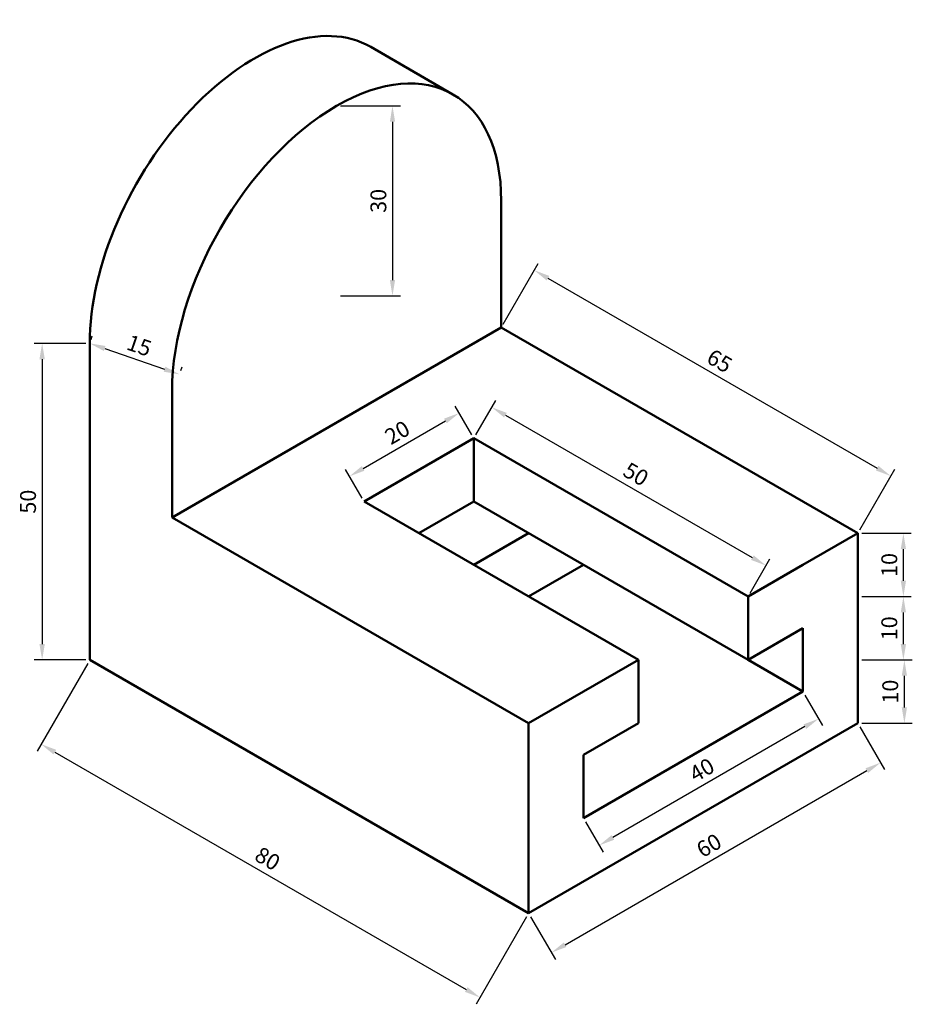
# Model space of a CAD drawing. Units: millimetres. Extents: x -12 to 129, y 4 to 160.
import ezdxf

# ---------------------------------------------------------------- set-up
doc = ezdxf.new("R2010")
doc.units = ezdxf.units.MM
doc.layers.add('M-DIMS', color=2, linetype='Continuous', lineweight=25)
doc.layers.add('M-OUTL', color=7, linetype='Continuous', lineweight=50)
doc.styles.get("Standard").update_dxf_attribs({"font": 'arial.ttf'})
doc.dimstyles.new('ISO-25', dxfattribs={"dimtxt": 2.5, "dimasz": 2.5, "dimexe": 1.25, "dimexo": 0.625, "dimtad": 1, "dimtxsty": 'Standard', "dimcen": 2.5, "dimadec": 0, "dimazin": 0, "dimtfac": 1, "dimtmove": 0, "dimatfit": 3, "dimfxl": 1, "dimarcsym": 0})

# ---------------------------------------------------------------- blocks, each defined once
blk = doc.blocks.new('*D1')
at = {"layer": 'Defpoints', "color": 0, "transparency": 16777216}
for p in [(37.82, 145.89), (37.82, 115.89), (46.64, 115.89)]:
    blk.add_point(p, dxfattribs=at)
at = {"layer": 'M-DIMS', "color": 0, "lineweight": -2, "transparency": 16777216}
for p, q in [((38.45, 145.89), (47.89, 145.89)), ((46.64, 143.39), (46.64, 118.39)), ((38.45, 115.89), (47.89, 115.89))]:
    blk.add_line(p, q, dxfattribs=at)
at = {"layer": 'M-DIMS', "color": 0, "transparency": 16777216}
for points in [[(46.23, 143.39), (47.06, 143.39), (46.64, 145.89)], [(46.23, 118.39), (47.06, 118.39), (46.64, 115.89)]]:
    blk.add_solid(points, dxfattribs=at)
at = {"layer": 'M-DIMS', "color": 0, "transparency": 16777216, "insert": (44.74, 130.89), "char_height": 2.5, "attachment_point": 5, "rotation": 90}
blk.add_mtext('30', dxfattribs=at)
blk = doc.blocks.new('*D2')
at = {"layer": 'Defpoints', "color": 0, "transparency": 16777216}
for p in [(63.8, 110.89), (125.31, 87.43), (120.1, 78.39)]:
    blk.add_point(p, dxfattribs=at)
at = {"layer": 'M-DIMS', "color": 0, "lineweight": -2, "transparency": 16777216}
for p, q in [((64.12, 111.43), (69.65, 121.01)), ((71.19, 118.68), (123.15, 88.68)), ((120.41, 78.93), (125.94, 88.51))]:
    blk.add_line(p, q, dxfattribs=at)
at = {"layer": 'M-DIMS', "color": 0, "transparency": 16777216}
for points in [[(71.4, 119.04), (70.98, 118.32), (69.02, 119.93)], [(123.36, 89.04), (122.94, 88.32), (125.31, 87.43)]]:
    blk.add_solid(points, dxfattribs=at)
at = {"layer": 'M-DIMS', "color": 0, "transparency": 16777216, "insert": (98.12, 105.33), "char_height": 2.5, "attachment_point": 5, "rotation": 330}
blk.add_mtext('65', dxfattribs=at)
blk = doc.blocks.new('*D3')
at = {"layer": 'Defpoints', "color": 0, "transparency": 16777216}
for p in [(120.1, 78.39), (127.29, 78.39), (120.1, 68.39)]:
    blk.add_point(p, dxfattribs=at)
at = {"layer": 'M-DIMS', "color": 0, "lineweight": -2, "transparency": 16777216}
for p, q in [((120.72, 78.39), (128.54, 78.39)), ((127.29, 70.89), (127.29, 75.89)), ((120.72, 68.39), (128.54, 68.39))]:
    blk.add_line(p, q, dxfattribs=at)
at = {"layer": 'M-DIMS', "color": 0, "transparency": 16777216}
for points in [[(126.87, 75.89), (127.71, 75.89), (127.29, 78.39)], [(126.87, 70.89), (127.71, 70.89), (127.29, 68.39)]]:
    blk.add_solid(points, dxfattribs=at)
at = {"layer": 'M-DIMS', "color": 0, "transparency": 16777216, "insert": (125.39, 73.39), "char_height": 2.5, "attachment_point": 5, "rotation": 90}
blk.add_mtext('10', dxfattribs=at)
blk = doc.blocks.new('*D4')
at = {"layer": 'Defpoints', "color": 0, "transparency": 16777216}
for p in [(120.1, 68.39), (127.29, 68.39), (120.1, 58.39)]:
    blk.add_point(p, dxfattribs=at)
at = {"layer": 'M-DIMS', "color": 0, "lineweight": -2, "transparency": 16777216}
for p, q in [((120.72, 68.39), (128.54, 68.39)), ((127.29, 60.89), (127.29, 65.89)), ((120.72, 58.39), (128.54, 58.39))]:
    blk.add_line(p, q, dxfattribs=at)
at = {"layer": 'M-DIMS', "color": 0, "transparency": 16777216}
for points in [[(126.87, 65.89), (127.71, 65.89), (127.29, 68.39)], [(126.87, 60.89), (127.71, 60.89), (127.29, 58.39)]]:
    blk.add_solid(points, dxfattribs=at)
at = {"layer": 'M-DIMS', "color": 0, "transparency": 16777216, "insert": (125.39, 63.39), "char_height": 2.5, "attachment_point": 5, "rotation": 90}
blk.add_mtext('10', dxfattribs=at)
blk = doc.blocks.new('*D5')
at = {"layer": 'Defpoints', "color": 0, "transparency": 16777216}
for p in [(120.1, 58.39), (127.45, 58.39), (120.1, 48.39)]:
    blk.add_point(p, dxfattribs=at)
at = {"layer": 'M-DIMS', "color": 0, "lineweight": -2, "transparency": 16777216}
for p, q in [((120.72, 58.39), (128.7, 58.39)), ((127.45, 50.89), (127.45, 55.89)), ((120.72, 48.39), (128.7, 48.39))]:
    blk.add_line(p, q, dxfattribs=at)
at = {"layer": 'M-DIMS', "color": 0, "transparency": 16777216}
for points in [[(127.03, 55.89), (127.86, 55.89), (127.45, 58.39)], [(127.03, 50.89), (127.86, 50.89), (127.45, 48.39)]]:
    blk.add_solid(points, dxfattribs=at)
at = {"layer": 'M-DIMS', "color": 0, "transparency": 16777216, "insert": (125.54, 53.39), "char_height": 2.5, "attachment_point": 5, "rotation": 90}
blk.add_mtext('10', dxfattribs=at)
blk = doc.blocks.new('*D6')
at = {"layer": 'Defpoints', "color": 0, "transparency": 16777216}
for p in [(120.1, 48.39), (123.69, 42.17), (68.13, 18.39)]:
    blk.add_point(p, dxfattribs=at)
at = {"layer": 'M-DIMS', "color": 0, "lineweight": -2, "transparency": 16777216}
for p, q in [((120.41, 47.85), (124.31, 41.09)), ((73.89, 13.42), (121.52, 40.92)), ((68.45, 17.85), (72.35, 11.09))]:
    blk.add_line(p, q, dxfattribs=at)
at = {"layer": 'M-DIMS', "color": 0, "transparency": 16777216}
for points in [[(121.31, 41.28), (121.73, 40.56), (123.69, 42.17)], [(73.68, 13.78), (74.1, 13.06), (71.73, 12.17)]]:
    blk.add_solid(points, dxfattribs=at)
at = {"layer": 'M-DIMS', "color": 0, "transparency": 16777216, "insert": (96.76, 28.82), "char_height": 2.5, "attachment_point": 5, "rotation": 30}
blk.add_mtext('60', dxfattribs=at)
blk = doc.blocks.new('*D7')
at = {"layer": 'Defpoints', "color": 0, "transparency": 16777216}
for p in [(111.44, 53.39), (76.79, 33.39), (79.27, 29.11)]:
    blk.add_point(p, dxfattribs=at)
at = {"layer": 'M-DIMS', "color": 0, "lineweight": -2, "transparency": 16777216}
for p, q in [((111.75, 52.85), (114.53, 48.03)), ((111.74, 47.86), (81.43, 30.36)), ((77.11, 32.85), (79.89, 28.03))]:
    blk.add_line(p, q, dxfattribs=at)
at = {"layer": 'M-DIMS', "color": 0, "transparency": 16777216}
for points in [[(111.53, 48.22), (111.95, 47.5), (113.91, 49.11)], [(81.22, 30.72), (81.64, 30), (79.27, 29.11)]]:
    blk.add_solid(points, dxfattribs=at)
at = {"layer": 'M-DIMS', "color": 0, "transparency": 16777216, "insert": (95.64, 40.75), "char_height": 2.5, "attachment_point": 5, "rotation": 30}
blk.add_mtext('40', dxfattribs=at)
blk = doc.blocks.new('*D8')
at = {"layer": 'Defpoints', "color": 0, "transparency": 16777216}
for p in [(59.47, 93.39), (105.61, 73.3), (102.78, 68.39)]:
    blk.add_point(p, dxfattribs=at)
at = {"layer": 'M-DIMS', "color": 0, "lineweight": -2, "transparency": 16777216}
for p, q in [((59.79, 93.93), (62.93, 99.38)), ((64.47, 97.05), (103.44, 74.55)), ((103.09, 68.93), (106.23, 74.38))]:
    blk.add_line(p, q, dxfattribs=at)
at = {"layer": 'M-DIMS', "color": 0, "transparency": 16777216}
for points in [[(64.68, 97.41), (64.26, 96.69), (62.31, 98.3)], [(103.65, 74.91), (103.24, 74.19), (105.61, 73.3)]]:
    blk.add_solid(points, dxfattribs=at)
at = {"layer": 'M-DIMS', "color": 0, "transparency": 16777216, "insert": (84.91, 87.45), "char_height": 2.5, "attachment_point": 5, "rotation": 330}
blk.add_mtext('50', dxfattribs=at)
blk = doc.blocks.new('*D9')
at = {"layer": 'Defpoints', "color": 0, "transparency": 16777216}
for p in [(57.17, 97.39), (59.47, 93.39), (42.15, 83.39)]:
    blk.add_point(p, dxfattribs=at)
at = {"layer": 'M-DIMS', "color": 0, "lineweight": -2, "transparency": 16777216}
for p, q in [((59.16, 93.93), (56.54, 98.47)), ((42.01, 88.64), (55, 96.14)), ((41.84, 83.93), (39.22, 88.47))]:
    blk.add_line(p, q, dxfattribs=at)
at = {"layer": 'M-DIMS', "color": 0, "transparency": 16777216}
for points in [[(54.79, 96.5), (55.21, 95.78), (57.17, 97.39)], [(41.8, 89), (42.22, 88.28), (39.85, 87.39)]]:
    blk.add_solid(points, dxfattribs=at)
at = {"layer": 'M-DIMS', "color": 0, "transparency": 16777216, "insert": (47.56, 94.03), "char_height": 2.5, "attachment_point": 5, "rotation": 30}
blk.add_mtext('20', dxfattribs=at)
blk = doc.blocks.new('*D10')
at = {"layer": 'Defpoints', "color": 0, "transparency": 16777216}
for p in [(-1.15, 58.39), (68.13, 18.39), (60.46, 5.09)]:
    blk.add_point(p, dxfattribs=at)
at = {"layer": 'M-DIMS', "color": 0, "lineweight": -2, "transparency": 16777216}
for p, q in [((-1.46, 57.85), (-9.45, 44.01)), ((-6.66, 43.84), (58.29, 6.34)), ((67.82, 17.85), (59.83, 4.01))]:
    blk.add_line(p, q, dxfattribs=at)
at = {"layer": 'M-DIMS', "color": 0, "transparency": 16777216}
for points in [[(-6.45, 44.21), (-6.87, 43.48), (-8.82, 45.09)], [(58.5, 6.71), (58.08, 5.98), (60.46, 5.09)]]:
    blk.add_solid(points, dxfattribs=at)
at = {"layer": 'M-DIMS', "color": 0, "transparency": 16777216, "insert": (26.77, 26.74), "char_height": 2.5, "attachment_point": 5, "rotation": 330}
blk.add_mtext('80', dxfattribs=at)
blk = doc.blocks.new('*D11')
at = {"layer": 'Defpoints', "color": 0, "transparency": 16777216}
for p in [(-1.15, 108.39), (13.03, 103.49), (13.03, 103.49)]:
    blk.add_point(p, dxfattribs=at)
at = {"layer": 'M-DIMS', "color": 0, "lineweight": -2, "transparency": 16777216}
for p, q in [((-0.94, 108.98), (-0.74, 109.57)), ((1.21, 107.57), (10.67, 104.31)), ((13.23, 104.08), (13.44, 104.67))]:
    blk.add_line(p, q, dxfattribs=at)
at = {"layer": 'M-DIMS', "color": 0, "transparency": 16777216}
for points in [[(1.35, 107.97), (1.08, 107.18), (-1.15, 108.39)], [(10.8, 104.7), (10.53, 103.91), (13.03, 103.49)]]:
    blk.add_solid(points, dxfattribs=at)
at = {"layer": 'M-DIMS', "color": 0, "transparency": 16777216, "insert": (6.56, 107.74), "char_height": 2.5, "attachment_point": 5, "rotation": 340.9288}
blk.add_mtext('15', dxfattribs=at)
blk = doc.blocks.new('*D12')
at = {"layer": 'Defpoints', "color": 0, "transparency": 16777216}
for p in [(-1.15, 108.39), (-8.66, 58.39), (-1.15, 58.39)]:
    blk.add_point(p, dxfattribs=at)
at = {"layer": 'M-DIMS', "color": 0, "lineweight": -2, "transparency": 16777216}
for p, q in [((-1.77, 108.39), (-9.91, 108.39)), ((-8.66, 105.89), (-8.66, 60.89)), ((-1.77, 58.39), (-9.91, 58.39))]:
    blk.add_line(p, q, dxfattribs=at)
at = {"layer": 'M-DIMS', "color": 0, "transparency": 16777216}
for points in [[(-9.08, 105.89), (-8.24, 105.89), (-8.66, 108.39)], [(-9.08, 60.89), (-8.24, 60.89), (-8.66, 58.39)]]:
    blk.add_solid(points, dxfattribs=at)
at = {"layer": 'M-DIMS', "color": 0, "transparency": 16777216, "insert": (-10.56, 83.39), "char_height": 2.5, "attachment_point": 5, "rotation": 90}
blk.add_mtext('50', dxfattribs=at)

msp = doc.modelspace()

# ---------------------------------------------------------------- linework, layer by layer
at = {"layer": 'M-OUTL'}
for p, q in [((56.194, 147.711), (43.204, 155.211)), ((63.804, 110.891), (63.804, 130.891)), ((11.842, 80.891), (63.804, 110.891)), ((63.804, 110.891), (120.096, 78.391)), ((-1.148, 58.391), (-1.148, 108.391)), ((-1.148, 58.391), (-1.148, 108.391)), ((11.842, 80.891), (11.842, 100.891)), ((42.153, 83.391), (59.474, 93.391)), ((59.474, 93.391), (102.775, 68.391)), ((59.474, 83.391), (59.474, 93.391)), ((85.455, 58.391), (42.153, 83.391)), ((50.813, 78.391), (59.473, 83.391)), ((102.775, 58.391), (59.474, 83.391)), ((68.134, 48.391), (11.842, 80.891)), ((59.474, 73.391), (68.134, 78.391)), ((120.096, 78.391), (111.435, 73.391)), ((120.096, 68.391), (120.096, 78.391)), ((68.134, 68.391), (76.794, 73.391)), ((111.435, 73.391), (102.775, 68.391)), ((102.775, 68.391), (102.775, 58.391)), ((120.096, 58.391), (120.096, 68.391)), ((102.775, 58.391), (111.435, 63.391)), ((111.435, 63.391), (111.435, 53.391)), ((68.134, 18.391), (-1.148, 58.391)), ((68.134, 48.391), (85.455, 58.391)), ((85.455, 48.391), (85.455, 58.391)), ((111.435, 53.391), (102.775, 58.391)), ((120.096, 48.391), (120.096, 58.391)), ((111.435, 53.391), (76.794, 33.391)), ((68.134, 18.391), (120.096, 48.391)), ((68.134, 18.391), (68.134, 48.391)), ((76.794, 43.391), (85.455, 48.391)), ((76.794, 33.391), (76.794, 43.391))]:
    msp.add_line(p, q, dxfattribs=at)
for centre, start_param in [((24.833, 123.391), 3.1415927), ((37.823, 115.891), 2.3561945)]:
    msp.add_ellipse(centre, major_axis=(-18.371, -31.82), ratio=0.5773503, start_param=start_param, end_param=5.4977871, dxfattribs=at)

# ---------------------------------------------------------------- dimensions: what is measured, and where the dimension line sits
at = {"layer": 'M-DIMS'}
for base, p1, p2, angle, override, picture, middle in [((46.644, 115.891), (37.823, 145.891), (37.823, 115.891), 90, {"dimclrd": 0, "dimclre": 0, "dimclrt": 0}, '*D1', (44.742, 130.891)), ((-8.66, 58.391), (-1.148, 108.391), (-1.148, 58.391), 270, {"dimrnd": 0}, '*D12', (-10.562, 83.391)), ((127.291, 78.391), (120.096, 68.391), (120.096, 78.391), 90, {"dimclrd": 0, "dimclre": 0, "dimclrt": 0}, '*D3', (125.389, 73.391)), ((127.291, 68.391), (120.096, 58.391), (120.096, 68.391), 90, {"dimclrd": 0, "dimclre": 0, "dimclrt": 0}, '*D4', (125.389, 63.391)), ((127.446, 58.391), (120.096, 48.391), (120.096, 58.391), 90, {"dimclrd": 0, "dimclre": 0, "dimclrt": 0}, '*D5', (125.545, 53.391))]:
    dim = msp.add_linear_dim(base=base, p1=p1, p2=p2, angle=angle, dimstyle='ISO-25', override=override, dxfattribs=at)
    dim.commit()
    dim.dimension.update_dxf_attribs({"geometry": picture, "text_midpoint": middle})
for p1, p2, distance, picture, middle in [((63.804, 110.891), (120.096, 78.391), 10.438, '*D2', (98.119, 105.327)), ((-1.148, 108.391), (13.029, 103.49), 0, '*D11', (6.562, 107.737)), ((42.153, 83.391), (59.474, 93.391), 4.613, '*D9', (47.556, 94.033)), ((59.474, 93.391), (102.775, 68.391), 5.667, '*D8', (84.909, 87.446)), ((-1.148, 58.391), (68.134, 18.391), -15.353, '*D10', (26.767, 26.742)), ((111.435, 53.391), (76.794, 33.391), 4.945, '*D7', (95.637, 40.755)), ((68.134, 18.391), (120.096, 48.391), -7.184, '*D6', (96.756, 28.816))]:
    dim = msp.add_aligned_dim(p1=p1, p2=p2, distance=distance, dimstyle='ISO-25', override={"dimclrd": 0, "dimclre": 0, "dimclrt": 0}, dxfattribs=at)
    dim.commit()
    dim.dimension.update_dxf_attribs({"geometry": picture, "text_midpoint": middle})

doc.saveas('drawing.dxf')
